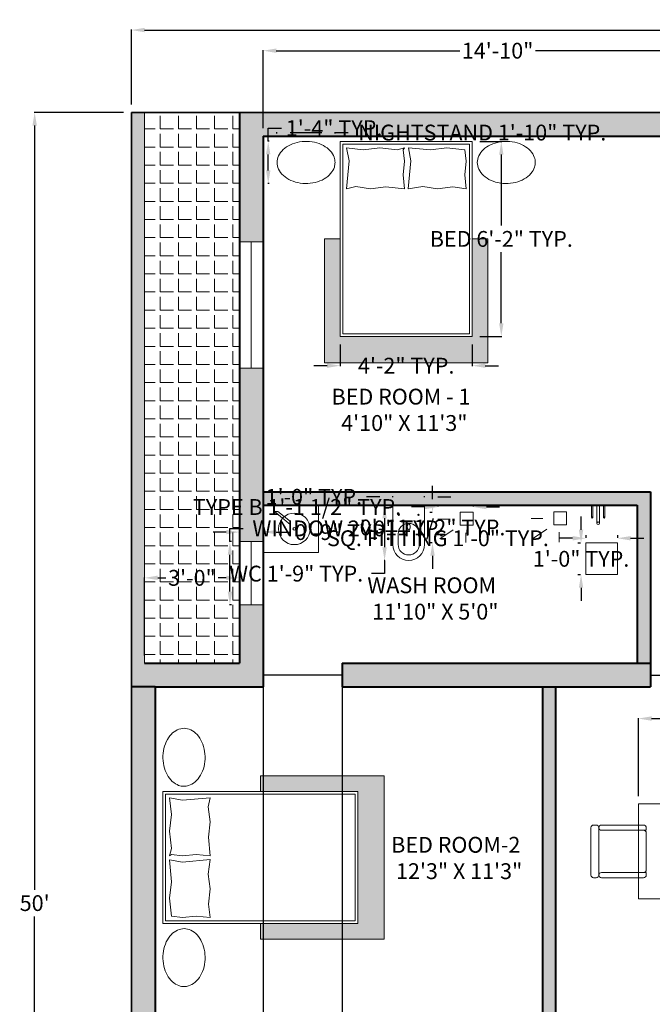
# Model space of a CAD drawing. Units: inches. Extents: x 242 to 808, y 202 to 873.
# Tile 2 of 3: x 242 to 482, y 500 to 873. Entities that reach past the tile are written whole.
import ezdxf

# ---------------------------------------------------------------- set-up
doc = ezdxf.new("R2010")
doc.units = ezdxf.units.IN
doc.header["$MEASUREMENT"] = 0
for name, color, linetype, lineweight in [('A-ANNO-DIMS', 2, 'Continuous', 18), ('A-AREA-IDEN', 7, 'Continuous', 25), ('A-DOOR', 3, 'Continuous', 25), ('A-FLOR-FIXT', 8, 'Continuous', 18), ('A-FURN', 8, 'Continuous', 18), ('A-FURN-PATT', 253, 'Continuous', 13), ('A-GLAZ', 4, 'Continuous', 18), ('A-SITE-PVMT', 8, 'Continuous', 18), ('A-SITE-PVMT-PATT', 254, 'Continuous', 13), ('A-WALL', 7, 'Continuous', 40), ('A-WALL-PATT', 30, 'Continuous', 13), ('C-PROP', 7, 'Continuous', 35)]:
    doc.layers.add(name, color=color, linetype=linetype, lineweight=lineweight)
doc.styles.get("Standard").update_dxf_attribs({"font": 'arial.ttf'})
doc.dimstyles.get("Standard").update_dxf_attribs({"dimtxt": 6, "dimasz": 5, "dimexe": 0.18, "dimexo": 3, "dimgap": 2, "dimtad": 0, "dimtih": 1, "dimtoh": 1, "dimdec": 0, "dimzin": 0, "dimdsep": 46, "dimlunit": 3, "dimtxsty": 'Standard', "dimcen": 0.09, "dimadec": 0, "dimazin": 0, "dimtfac": 1, "dimtdec": 0, "dimtofl": 0, "dimtmove": 0, "dimatfit": 3, "dimfxl": 1, "dimtolj": 1, "dimtzin": 0, "dimarcsym": 0})

# ---------------------------------------------------------------- blocks, each defined once
blk = doc.blocks.new('*D7')
at = {"layer": 'A-ANNO-DIMS', "color": 0, "lineweight": -2, "transparency": 16777216}
for p, q in [((284.66, 841.15), (284.66, 869.56)), ((289.66, 869.38), (517.45, 869.38)), ((759.66, 869.38), (531.88, 869.38)), ((764.66, 841.15), (764.66, 869.56))]:
    blk.add_line(p, q, dxfattribs=at)
at = {"layer": 'A-ANNO-DIMS', "color": 0, "transparency": 16777216}
for points in [[(289.66, 870.21), (289.66, 868.54), (284.66, 869.38)], [(759.66, 870.21), (759.66, 868.54), (764.66, 869.38)]]:
    blk.add_solid(points, dxfattribs=at)
at = {"layer": 'Defpoints', "color": 0, "transparency": 16777216}
for p in [(764.66, 869.38), (284.66, 838.15), (764.66, 838.15)]:
    blk.add_point(p, dxfattribs=at)
at = {"layer": 'A-ANNO-DIMS', "color": 0, "transparency": 16777216, "insert": (524.66, 869.38), "char_height": 6, "attachment_point": 5}
blk.add_mtext("\\A1;40'", dxfattribs=at)
blk = doc.blocks.new('*D8')
at = {"layer": 'A-ANNO-DIMS', "color": 0, "lineweight": -2, "transparency": 16777216}
for p, q in [((281.66, 838.15), (247.79, 838.15)), ((247.97, 833.15), (247.97, 543.22)), ((247.97, 243.15), (247.97, 533.09)), ((281.66, 238.15), (247.79, 238.15))]:
    blk.add_line(p, q, dxfattribs=at)
at = {"layer": 'A-ANNO-DIMS', "color": 0, "transparency": 16777216}
for points in [[(247.13, 833.15), (248.8, 833.15), (247.97, 838.15)], [(247.13, 243.15), (248.8, 243.15), (247.97, 238.15)]]:
    blk.add_solid(points, dxfattribs=at)
at = {"layer": 'Defpoints', "color": 0, "transparency": 16777216}
for p in [(284.66, 838.15), (247.97, 238.15), (284.66, 238.15)]:
    blk.add_point(p, dxfattribs=at)
at = {"layer": 'A-ANNO-DIMS', "color": 0, "transparency": 16777216, "insert": (247.97, 538.15), "char_height": 6, "attachment_point": 5}
blk.add_mtext("\\A1;50'", dxfattribs=at)
blk = doc.blocks.new('DINING-CHAIR')
for p, q in [((2, 18), (2, 20)), ((3, 21), (17, 21)), ((18, 21), (18, 18)), ((19, 21), (18, 21)), ((18, 20), (18, 18)), ((20, 4), (20, 20)), ((1, 0), (10, 0)), ((10, 0), (19, 0))]:
    blk.add_line(p, q)
for points in [[(0, 1), (0, 2, -0.414214), (1, 3), (1, 3, 0.414214), (2, 4), (2, 21), (1, 21, 0.414214), (0, 20), (0, 4, 0.414214), (1, 3), (19, 3)], [(18, 18), (18, 4, 0.414214), (19, 3), (19, 3, -0.414214), (20, 2), (20, 1)]]:
    blk.add_lwpolyline(points, format="xyb")
for centre, start, end in [((3, 20), 90, 180), ((17, 20), 0, 90), ((19, 20), 0, 90), ((19, 4), 270, 0), ((1, 1), 180, 270), ((19, 1), 270, 0)]:
    blk.add_arc(centre, 1, start, end)
blk = doc.blocks.new('BED-DOUBLE')
for p, q in [((2.42, 71.51), (8.74, 70.74)), ((3.32, 66.6), (2.42, 71.51)), ((2.42, 71.51), (2.42, 71.51)), ((8.74, 70.74), (15, 71.51)), ((15, 71.51), (21.65, 70.74)), ((21.65, 70.74), (24.42, 71.51)), ((24.42, 71.51), (23.82, 70.81)), ((25.88, 71.51), (34.2, 70.74)), ((26.78, 66.6), (25.88, 71.51)), ((25.88, 71.51), (25.88, 71.51)), ((34.2, 70.74), (40.46, 71.51)), ((40.46, 71.51), (47.28, 70.81)), ((23.82, 70.81), (24.35, 66.53)), ((47.28, 70.81), (47.81, 66.53)), ((2.35, 56.03), (3.32, 66.6)), ((24.35, 66.53), (23.85, 61.36)), ((25.81, 56.03), (26.78, 66.6)), ((47.81, 66.53), (47.32, 61.36)), ((23.85, 61.36), (24.35, 56.03)), ((47.32, 61.36), (47.81, 56.03)), ((5.85, 56.87), (2.35, 56.03)), ((11.48, 56.03), (5.85, 56.87)), ((17.24, 56.78), (11.48, 56.03)), ((24.35, 56.03), (17.24, 56.78)), ((31.31, 56.87), (25.81, 56.03)), ((36.94, 56.03), (31.31, 56.87)), ((42.7, 56.78), (36.94, 56.03)), ((47.81, 56.03), (42.7, 56.78))]:
    blk.add_line(p, q)
for points in [[(0, 74), (50, 74), (50, 0), (0, 0)], [(1, 73), (49, 73), (49, 1), (1, 1)]]:
    blk.add_lwpolyline(points, close=True)
blk = doc.blocks.new('BEDSIDE-TABLE')
blk.add_open_spline([(22, 8), (22, 8.68), (21.88, 9.37), (21.33, 10.88), (20.82, 11.7), (19.44, 13.19), (18.57, 13.86), (16.55, 14.96), (15.4, 15.38), (12.98, 15.92), (11.7, 16.04), (9.16, 15.94), (7.91, 15.73), (5.57, 15.01), (4.5, 14.5), (2.65, 13.27), (1.88, 12.54), (0.72, 10.97), (0.33, 10.13), (-0.05, 8.41), (-0.05, 7.54), (0.35, 5.81), (0.76, 4.96), (1.95, 3.37), (2.75, 2.64), (4.64, 1.41), (5.75, 0.92), (8.13, 0.22), (9.41, 0.03), (11.98, -0.02), (13.27, 0.12), (15.7, 0.71), (16.84, 1.17), (18.83, 2.32), (19.68, 3.02), (21, 4.56), (21.47, 5.4), (21.91, 6.84), (22, 7.42), (22, 8)], degree=3, knots=[0, 0, 0, 0, 0.267442, 0.267442, 0.605946, 0.605946, 0.944449, 0.944449, 1.282952, 1.282952, 1.621455, 1.621455, 1.959959, 1.959959, 2.298462, 2.298462, 2.636965, 2.636965, 2.975469, 2.975469, 3.313972, 3.313972, 3.656728, 3.656728, 3.999485, 3.999485, 4.342242, 4.342242, 4.684998, 4.684998, 5.027755, 5.027755, 5.370511, 5.370511, 5.713268, 5.713268, 6.056024, 6.056024, 6.283185, 6.283185, 6.283185, 6.283185])
blk = doc.blocks.new('LAVATORY-VANITY')
for p, q in [((15.59, 16.67), (10.6, 10.67)), ((11.73, 10.63), (15.59, 15.35)), ((15.59, 16.67), (15.59, 15.35)), ((10.6, 10.67), (11.73, 10.63))]:
    blk.add_line(p, q)
blk.add_lwpolyline([(0, 21), (18, 21), (18, 0), (0, 0)], close=True)
for radius in [6, 0.5]:
    blk.add_circle((8.99, 9.16), radius)
blk = doc.blocks.new('WC-PAN')
for p, q in [((0, 15), (0, 0)), ((12, 0), (12, 15)), ((2, 14.93), (2, 10.93)), ((10, 14.93), (10, 10.93))]:
    blk.add_line(p, q)
for centre, radius, start, end in [((6, 15), 6, 0, 180), ((6, 14.93), 4, 0, 180), ((6, 10.93), 4, 180, 0)]:
    blk.add_arc(centre, radius, start, end)
blk.add_ellipse((6, 8.26), major_axis=(0, 1.09), ratio=0.500408)
blk = doc.blocks.new('SHOWER-MIXER')
for p, q in [((0, 4.4), (0, 0)), ((0.5, 4.4), (0.5, 0)), ((2, 6.9), (2, 0)), ((3, 6.9), (3, 0)), ((4.5, 4.4), (4.5, 0)), ((5, 4.4), (5, 0))]:
    blk.add_line(p, q)
for centre, radius in [((0.25, 4.65), 0.25), ((2.5, 6.9), 0.5), ((4.75, 4.65), 0.25)]:
    blk.add_circle(centre, radius)
blk = doc.blocks.new('BATH-FITTING-B')
for p, q in [((2.85, 7.76), (2.85, 11.5)), ((7.55, 6.61), (12.62, 10.02)), ((9.01, 2.54), (13.42, 2.54))]:
    blk.add_line(p, q)
blk.add_lwpolyline([(0, 4.89), (4.89, 4.89), (4.89, 0), (0, 0)], close=True)
blk = doc.blocks.new('WIN-24IN')
blk.add_line((4.5, 24), (4.5, 0))
blk.add_lwpolyline([(0, 24), (9, 24), (9, 0), (0, 0)], close=True)
blk = doc.blocks.new('WIN-48IN')
blk.add_line((4.5, 48), (4.5, 0))
blk.add_lwpolyline([(0, 48), (9, 48), (9, 0), (0, 0)], close=True)
blk = doc.blocks.new('DOOR-30IN-PLAN')
blk.add_line((0, 30), (0, 0))
blk = doc.blocks.new('BATH-FITTING-12IN-SQ')
blk.add_lwpolyline([(0, 12), (12, 12), (12, 0), (0, 0)], close=True)
blk = doc.blocks.new('*D21')
at = {"layer": 'A-ANNO-DIMS', "color": 0, "lineweight": -2, "transparency": 16777216}
for p, q in [((416.96, 827.14), (425.24, 827.14)), ((425.06, 822.14), (425.06, 795.21)), ((425.06, 758.14), (425.06, 785.08)), ((416.96, 753.14), (425.24, 753.14))]:
    blk.add_line(p, q, dxfattribs=at)
at = {"layer": 'A-ANNO-DIMS', "color": 0, "transparency": 16777216}
for points in [[(424.22, 822.14), (425.89, 822.14), (425.06, 827.14)], [(424.22, 758.14), (425.89, 758.14), (425.06, 753.14)]]:
    blk.add_solid(points, dxfattribs=at)
at = {"layer": 'Defpoints', "color": 0, "transparency": 16777216}
for p in [(413.96, 827.14), (425.06, 827.14), (413.96, 753.14)]:
    blk.add_point(p, dxfattribs=at)
at = {"layer": 'A-ANNO-DIMS', "color": 0, "transparency": 16777216, "insert": (425.06, 790.14), "char_height": 6, "attachment_point": 5}
blk.add_mtext('\\A1;BED 6\'-2" TYP.', dxfattribs=at)
blk = doc.blocks.new('*D22')
at = {"layer": 'A-ANNO-DIMS', "color": 0, "lineweight": -2, "transparency": 16777216}
for p, q in [((363.96, 750.14), (363.96, 741.86)), ((413.96, 750.14), (413.96, 741.86)), ((358.96, 742.04), (353.96, 742.04)), ((418.96, 742.04), (423.96, 742.04))]:
    blk.add_line(p, q, dxfattribs=at)
at = {"layer": 'A-ANNO-DIMS', "color": 0, "transparency": 16777216}
for points in [[(358.96, 742.88), (358.96, 741.21), (363.96, 742.04)], [(418.96, 742.88), (418.96, 741.21), (413.96, 742.04)]]:
    blk.add_solid(points, dxfattribs=at)
at = {"layer": 'Defpoints', "color": 0, "transparency": 16777216}
for p in [(363.96, 753.14), (413.96, 753.14), (413.96, 742.04)]:
    blk.add_point(p, dxfattribs=at)
at = {"layer": 'A-ANNO-DIMS', "color": 0, "transparency": 16777216, "insert": (388.96, 742.04), "char_height": 6, "attachment_point": 5}
blk.add_mtext('\\A1;4\'-2" TYP.', dxfattribs=at)
blk = doc.blocks.new('*D23')
at = {"layer": 'A-ANNO-DIMS', "color": 0, "lineweight": -2, "transparency": 16777216}
for p, q in [((339.9, 830.18), (339.9, 830.67)), ((344.9, 830.49), (356.96, 830.49)), ((361.96, 830.18), (361.96, 830.67)), ((361.96, 830.49), (366.96, 830.49))]:
    blk.add_line(p, q, dxfattribs=at)
at = {"layer": 'A-ANNO-DIMS', "color": 0, "transparency": 16777216}
for points in [[(344.9, 831.33), (344.9, 829.66), (339.9, 830.49)], [(356.96, 831.33), (356.96, 829.66), (361.96, 830.49)]]:
    blk.add_solid(points, dxfattribs=at)
at = {"layer": 'Defpoints', "color": 0, "transparency": 16777216}
for p in [(361.96, 830.49), (339.9, 827.18), (361.96, 827.18)]:
    blk.add_point(p, dxfattribs=at)
at = {"layer": 'A-ANNO-DIMS', "color": 0, "transparency": 16777216, "insert": (417.83, 830.49), "char_height": 6, "attachment_point": 5}
blk.add_mtext('\\A1;NIGHTSTAND 1\'-10" TYP.', dxfattribs=at)
blk = doc.blocks.new('*D24')
at = {"layer": 'A-ANNO-DIMS', "color": 0, "lineweight": -2, "transparency": 16777216}
for p, q in [((336.6, 827.18), (336.6, 832.18)), ((336.6, 832.18), (341.6, 832.18)), ((336.9, 827.18), (336.42, 827.18)), ((336.6, 816.12), (336.6, 822.18)), ((336.9, 811.12), (336.42, 811.12))]:
    blk.add_line(p, q, dxfattribs=at)
at = {"layer": 'A-ANNO-DIMS', "color": 0, "transparency": 16777216}
for points in [[(335.76, 822.18), (337.43, 822.18), (336.6, 827.18)], [(335.76, 816.12), (337.43, 816.12), (336.6, 811.12)]]:
    blk.add_solid(points, dxfattribs=at)
at = {"layer": 'Defpoints', "color": 0, "transparency": 16777216}
for p in [(336.6, 827.18), (339.9, 827.18), (339.9, 811.12)]:
    blk.add_point(p, dxfattribs=at)
at = {"layer": 'A-ANNO-DIMS', "color": 0, "transparency": 16777216, "insert": (361.6, 832.18), "char_height": 6, "attachment_point": 5}
blk.add_mtext('\\A1;1\'-4" TYP.', dxfattribs=at)
blk = doc.blocks.new('*D29')
at = {"layer": 'A-ANNO-DIMS', "color": 0, "lineweight": -2, "transparency": 16777216}
for p, q in [((380.91, 689.15), (380.58, 689.15)), ((380.76, 684.15), (380.76, 673.15)), ((380.91, 668.15), (380.58, 668.15)), ((380.76, 668.15), (380.76, 663.15)), ((380.76, 663.15), (375.76, 663.15))]:
    blk.add_line(p, q, dxfattribs=at)
at = {"layer": 'A-ANNO-DIMS', "color": 0, "transparency": 16777216}
for points in [[(379.93, 684.15), (381.6, 684.15), (380.76, 689.15)], [(379.93, 673.15), (381.6, 673.15), (380.76, 668.15)]]:
    blk.add_solid(points, dxfattribs=at)
at = {"layer": 'Defpoints', "color": 0, "transparency": 16777216}
for p in [(383.91, 689.15), (380.76, 668.15), (383.91, 668.15)]:
    blk.add_point(p, dxfattribs=at)
at = {"layer": 'A-ANNO-DIMS', "color": 0, "transparency": 16777216, "insert": (347.21, 663.15), "char_height": 6, "attachment_point": 5}
blk.add_mtext('\\A1;WC 1\'-9" TYP.', dxfattribs=at)
blk = doc.blocks.new('*D30')
at = {"layer": 'A-ANNO-DIMS', "color": 0, "lineweight": -2, "transparency": 16777216}
for p, q in [((378.91, 692.3), (373.91, 692.3)), ((383.91, 692.15), (383.91, 692.48)), ((395.91, 692.15), (395.91, 692.48)), ((400.91, 692.3), (405.91, 692.3))]:
    blk.add_line(p, q, dxfattribs=at)
at = {"layer": 'A-ANNO-DIMS', "color": 0, "transparency": 16777216}
for points in [[(378.91, 693.14), (378.91, 691.47), (383.91, 692.3)], [(400.91, 693.14), (400.91, 691.47), (395.91, 692.3)]]:
    blk.add_solid(points, dxfattribs=at)
at = {"layer": 'Defpoints', "color": 0, "transparency": 16777216}
for p in [(383.91, 692.3), (383.91, 689.15), (395.91, 689.15)]:
    blk.add_point(p, dxfattribs=at)
at = {"layer": 'A-ANNO-DIMS', "color": 0, "transparency": 16777216, "insert": (353.91, 692.3), "char_height": 6, "attachment_point": 5}
blk.add_mtext('\\A1;1\'-0" TYP.', dxfattribs=at)
blk = doc.blocks.new('*D35')
at = {"layer": 'A-ANNO-DIMS', "color": 0, "lineweight": -2, "transparency": 16777216}
for p, q in [((395.97, 688.43), (390.97, 688.43)), ((400.97, 689.42), (400.97, 688.61)), ((414.39, 689.42), (414.39, 688.61)), ((419.39, 688.43), (424.39, 688.43))]:
    blk.add_line(p, q, dxfattribs=at)
at = {"layer": 'A-ANNO-DIMS', "color": 0, "transparency": 16777216}
for points in [[(395.97, 689.26), (395.97, 687.59), (400.97, 688.43)], [(419.39, 689.26), (419.39, 687.59), (414.39, 688.43)]]:
    blk.add_solid(points, dxfattribs=at)
at = {"layer": 'Defpoints', "color": 0, "transparency": 16777216}
for p in [(400.97, 688.43), (400.97, 686.42), (414.39, 686.42)]:
    blk.add_point(p, dxfattribs=at)
at = {"layer": 'A-ANNO-DIMS', "color": 0, "transparency": 16777216, "insert": (347.54, 688.43), "char_height": 6, "attachment_point": 5}
blk.add_mtext('\\A1;TYPE B 1\'-1 1/2" TYP.', dxfattribs=at)
blk = doc.blocks.new('*D36')
at = {"layer": 'A-ANNO-DIMS', "color": 0, "lineweight": -2, "transparency": 16777216}
for p, q in [((398.95, 691.42), (398.95, 696.42)), ((397.97, 686.42), (398.77, 686.42)), ((397.97, 674.91), (398.77, 674.91)), ((398.95, 669.91), (398.95, 664.91))]:
    blk.add_line(p, q, dxfattribs=at)
at = {"layer": 'A-ANNO-DIMS', "color": 0, "transparency": 16777216}
for points in [[(398.12, 691.42), (399.79, 691.42), (398.95, 686.42)], [(398.12, 669.91), (399.79, 669.91), (398.95, 674.91)]]:
    blk.add_solid(points, dxfattribs=at)
at = {"layer": 'Defpoints', "color": 0, "transparency": 16777216}
for p in [(400.97, 686.42), (398.95, 674.91), (400.97, 674.91)]:
    blk.add_point(p, dxfattribs=at)
at = {"layer": 'A-ANNO-DIMS', "color": 0, "transparency": 16777216, "insert": (398.95, 680.66), "char_height": 6, "attachment_point": 5}
blk.add_mtext('\\A1;0\'-11 1/2" TYP.', dxfattribs=at)
blk = doc.blocks.new('*D37')
at = {"layer": 'A-ANNO-DIMS', "color": 0, "lineweight": -2, "transparency": 16777216}
for p, q in [((452.13, 676.57), (447.13, 676.57)), ((457.13, 677.77), (457.13, 676.75)), ((469.13, 677.77), (469.13, 676.75)), ((474.13, 676.57), (479.13, 676.57))]:
    blk.add_line(p, q, dxfattribs=at)
at = {"layer": 'A-ANNO-DIMS', "color": 0, "transparency": 16777216}
for points in [[(452.13, 677.4), (452.13, 675.74), (457.13, 676.57)], [(474.13, 677.4), (474.13, 675.74), (469.13, 676.57)]]:
    blk.add_solid(points, dxfattribs=at)
at = {"layer": 'Defpoints', "color": 0, "transparency": 16777216}
for p in [(457.13, 676.57), (457.13, 674.77), (469.13, 674.77)]:
    blk.add_point(p, dxfattribs=at)
at = {"layer": 'A-ANNO-DIMS', "color": 0, "transparency": 16777216, "insert": (401.01, 676.57), "char_height": 6, "attachment_point": 5}
blk.add_mtext('\\A1;SQ. FITTING 1\'-0" TYP.', dxfattribs=at)
blk = doc.blocks.new('*D38')
at = {"layer": 'A-ANNO-DIMS', "color": 0, "lineweight": -2, "transparency": 16777216}
for p, q in [((455.33, 679.77), (455.33, 684.77)), ((454.13, 674.77), (455.15, 674.77)), ((454.13, 662.77), (455.15, 662.77)), ((455.33, 657.77), (455.33, 652.77))]:
    blk.add_line(p, q, dxfattribs=at)
at = {"layer": 'A-ANNO-DIMS', "color": 0, "transparency": 16777216}
for points in [[(454.49, 679.77), (456.16, 679.77), (455.33, 674.77)], [(454.49, 657.77), (456.16, 657.77), (455.33, 662.77)]]:
    blk.add_solid(points, dxfattribs=at)
at = {"layer": 'Defpoints', "color": 0, "transparency": 16777216}
for p in [(457.13, 674.77), (455.33, 662.77), (457.13, 662.77)]:
    blk.add_point(p, dxfattribs=at)
at = {"layer": 'A-ANNO-DIMS', "color": 0, "transparency": 16777216, "insert": (455.33, 668.77), "char_height": 6, "attachment_point": 5}
blk.add_mtext('\\A1;1\'-0" TYP.', dxfattribs=at)
blk = doc.blocks.new('*D39')
at = {"layer": 'A-ANNO-DIMS', "color": 0, "lineweight": -2, "transparency": 16777216}
for p, q in [((322.06, 675.31), (322.06, 680.31)), ((322.06, 680.31), (327.06, 680.31)), ((322.66, 675.31), (321.88, 675.31)), ((322.06, 656.31), (322.06, 670.31)), ((322.66, 651.31), (321.88, 651.31))]:
    blk.add_line(p, q, dxfattribs=at)
at = {"layer": 'A-ANNO-DIMS', "color": 0, "transparency": 16777216}
for points in [[(321.23, 670.31), (322.9, 670.31), (322.06, 675.31)], [(321.23, 656.31), (322.9, 656.31), (322.06, 651.31)]]:
    blk.add_solid(points, dxfattribs=at)
at = {"layer": 'Defpoints', "color": 0, "transparency": 16777216}
for p in [(322.06, 675.31), (325.66, 675.31), (325.66, 651.31)]:
    blk.add_point(p, dxfattribs=at)
at = {"layer": 'A-ANNO-DIMS', "color": 0, "transparency": 16777216, "insert": (367.03, 680.31), "char_height": 6, "attachment_point": 5}
blk.add_mtext('\\A1;WINDOW 2\'-0" TYP.', dxfattribs=at)
blk = doc.blocks.new('*D40')
at = {"layer": 'A-ANNO-DIMS', "color": 0, "lineweight": -2, "transparency": 16777216}
for p, q in [((320.66, 678.91), (315.66, 678.91)), ((325.66, 678.31), (325.66, 679.09)), ((334.66, 678.31), (334.66, 679.09)), ((339.66, 678.91), (344.66, 678.91))]:
    blk.add_line(p, q, dxfattribs=at)
at = {"layer": 'A-ANNO-DIMS', "color": 0, "transparency": 16777216}
for points in [[(320.66, 679.75), (320.66, 678.08), (325.66, 678.91)], [(339.66, 679.75), (339.66, 678.08), (334.66, 678.91)]]:
    blk.add_solid(points, dxfattribs=at)
at = {"layer": 'Defpoints', "color": 0, "transparency": 16777216}
for p in [(334.66, 678.91), (325.66, 675.31), (334.66, 675.31)]:
    blk.add_point(p, dxfattribs=at)
at = {"layer": 'A-ANNO-DIMS', "color": 0, "transparency": 16777216, "insert": (364.95, 678.91), "char_height": 6, "attachment_point": 5}
blk.add_mtext('\\A1;0\'-9" TYP.', dxfattribs=at)
blk = doc.blocks.new('*D43')
at = {"layer": 'A-ANNO-DIMS', "color": 0, "lineweight": -2, "transparency": 16777216}
for p, q in [((334.66, 832.15), (334.66, 861.73)), ((339.66, 861.55), (409.31, 861.55)), ((507.66, 861.55), (438.02, 861.55)), ((512.66, 832.15), (512.66, 861.73))]:
    blk.add_line(p, q, dxfattribs=at)
at = {"layer": 'A-ANNO-DIMS', "color": 0, "transparency": 16777216}
for points in [[(339.66, 862.39), (339.66, 860.72), (334.66, 861.55)], [(507.66, 862.39), (507.66, 860.72), (512.66, 861.55)]]:
    blk.add_solid(points, dxfattribs=at)
at = {"layer": 'Defpoints', "color": 0, "transparency": 16777216}
for p in [(512.66, 861.55), (334.66, 829.15), (512.66, 829.15)]:
    blk.add_point(p, dxfattribs=at)
at = {"layer": 'A-ANNO-DIMS', "color": 0, "transparency": 16777216, "insert": (423.66, 861.55), "char_height": 6, "attachment_point": 5}
blk.add_mtext('\\A1;14\'-10"', dxfattribs=at)
blk = doc.blocks.new('*D46')
at = {"layer": 'A-ANNO-DIMS', "color": 0, "lineweight": -2, "transparency": 16777216}
for p, q in [((364.66, 626.15), (364.66, 205.57)), ((334.66, 621.65), (334.66, 205.57)), ((329.66, 205.75), (324.66, 205.75)), ((369.66, 205.75), (374.66, 205.75))]:
    blk.add_line(p, q, dxfattribs=at)
at = {"layer": 'A-ANNO-DIMS', "color": 0, "transparency": 16777216}
for points in [[(329.66, 206.59), (329.66, 204.92), (334.66, 205.75)], [(369.66, 206.59), (369.66, 204.92), (364.66, 205.75)]]:
    blk.add_solid(points, dxfattribs=at)
at = {"layer": 'Defpoints', "color": 0, "transparency": 16777216}
for p in [(364.66, 629.15), (334.66, 624.65), (364.66, 205.75)]:
    blk.add_point(p, dxfattribs=at)
at = {"layer": 'A-ANNO-DIMS', "color": 0, "transparency": 16777216, "insert": (349.66, 205.75), "char_height": 6, "attachment_point": 5}
blk.add_mtext('\\A1;2\'-6"', dxfattribs=at)
blk = doc.blocks.new('*D49')
at = {"layer": 'A-ANNO-DIMS', "color": 0, "lineweight": -2, "transparency": 16777216}
for p, q in [((289.66, 632.15), (289.66, 661.73)), ((294.66, 661.55), (297.69, 661.55)), ((320.66, 661.55), (317.64, 661.55)), ((325.66, 632.15), (325.66, 661.73))]:
    blk.add_line(p, q, dxfattribs=at)
at = {"layer": 'A-ANNO-DIMS', "color": 0, "transparency": 16777216}
for points in [[(294.66, 662.39), (294.66, 660.72), (289.66, 661.55)], [(320.66, 662.39), (320.66, 660.72), (325.66, 661.55)]]:
    blk.add_solid(points, dxfattribs=at)
at = {"layer": 'Defpoints', "color": 0, "transparency": 16777216}
for p in [(325.66, 661.55), (289.66, 629.15), (325.66, 629.15)]:
    blk.add_point(p, dxfattribs=at)
at = {"layer": 'A-ANNO-DIMS', "color": 0, "transparency": 16777216, "insert": (307.66, 661.55), "char_height": 6, "attachment_point": 5}
blk.add_mtext('\\A1;3\'-0"', dxfattribs=at)
blk = doc.blocks.new('*D50')
at = {"layer": 'A-ANNO-DIMS', "color": 0, "lineweight": -2, "transparency": 16777216}
for p, q in [((477.06, 578.76), (477.06, 608.34)), ((482.06, 608.16), (515.08, 608.16)), ((568.06, 608.16), (535.04, 608.16)), ((573.06, 578.76), (573.06, 608.34))]:
    blk.add_line(p, q, dxfattribs=at)
at = {"layer": 'A-ANNO-DIMS', "color": 0, "transparency": 16777216}
for points in [[(482.06, 608.99), (482.06, 607.32), (477.06, 608.16)], [(568.06, 608.99), (568.06, 607.32), (573.06, 608.16)]]:
    blk.add_solid(points, dxfattribs=at)
at = {"layer": 'Defpoints', "color": 0, "transparency": 16777216}
for p in [(573.06, 608.16), (477.06, 575.76), (573.06, 575.76)]:
    blk.add_point(p, dxfattribs=at)
at = {"layer": 'A-ANNO-DIMS', "color": 0, "transparency": 16777216, "insert": (525.06, 608.16), "char_height": 6, "attachment_point": 5}
blk.add_mtext('\\A1;8\'-0"', dxfattribs=at)

msp = doc.modelspace()

# ---------------------------------------------------------------- hatches: boundary and pattern name
at = {"layer": 'A-FURN-PATT'}
h = msp.add_hatch(dxfattribs=at)
h.set_pattern_fill('AR-SAND', color=256, scale=2, angle=180)
h.paths.add_polyline_path([(380.66, 586.46), (333.66, 586.46), (333.66, 580.46), (370.66, 580.46), (370.66, 530.46), (333.66, 530.46), (333.66, 524.46), (370.66, 524.46), (380.66, 524.46)])
h.paths.add_polyline_path([(419.96, 753.14), (419.96, 790.14), (413.96, 790.14), (413.96, 753.14), (363.95, 753.14), (363.95, 790.14), (357.96, 790.14), (357.96, 743.14), (419.96, 743.14)])
at = {"layer": 'A-SITE-PVMT-PATT'}
h = msp.add_hatch(dxfattribs=at)
h.set_pattern_fill('ANGLE', color=256, scale=25)
h.set_pattern_definition([(0, (0, 0), (0, 6.875), [5, -1.875]), (90, (0, 0), (-6.875, 4e-16), [5, -1.875])])
h.paths.add_polyline_path([(325.66, 838.15), (289.66, 838.15), (289.66, 629.15), (325.66, 629.15)])
at = {"layer": 'A-WALL-PATT'}
h = msp.add_hatch(color=256, dxfattribs=at)
h.dxf.hatch_style = 1
h.paths.add_polyline_path([(521.66, 838.15), (325.66, 838.15), (325.66, 789.05), (334.66, 789.05), (334.66, 829.15), (512.66, 829.15), (512.66, 788.15), (714.66, 788.15), (723.66, 788.15), (723.66, 797.15), (521.66, 797.15)])
h.paths.add_polyline_path([(764.66, 838.15), (521.66, 838.15), (521.66, 833.15), (759.66, 833.15), (759.66, 629.15), (764.66, 629.15)])
h.paths.add_polyline_path([(723.66, 788.15), (714.66, 788.15), (714.66, 767.17), (723.66, 767.17)], flags=17)
h.paths.add_polyline_path([(723.66, 743.17), (714.66, 743.17), (714.66, 721.15), (622.66, 721.15), (622.66, 758.15), (617.66, 758.15), (617.66, 721.15), (521.66, 721.15), (521.66, 716.15), (643.66, 716.15), (643.66, 659.15), (648.66, 659.15), (648.66, 716.15), (714.66, 716.15), (714.66, 688.28), (723.66, 688.28)], flags=17)
h.paths.add_polyline_path([(764.66, 629.15), (759.66, 629.15), (723.66, 629.15), (723.66, 664.28), (714.66, 664.28), (714.66, 629.15), (648.66, 629.15), (643.66, 629.15), (643.66, 620.15), (759.66, 620.15), (759.66, 403.15), (759.66, 398.15), (759.66, 238.15), (764.66, 238.15)])
h.paths.add_polyline_path([(521.66, 758.15), (512.66, 758.15), (512.66, 620.15), (521.66, 620.15)])
h.paths.add_polyline_path([(481.66, 694.15), (334.66, 694.15), (334.66, 689.15), (476.66, 689.15), (476.66, 629.15), (481.66, 629.15)])
h.paths.add_polyline_path([(334.66, 741.05), (325.66, 741.05), (325.66, 675.31), (334.66, 675.31), (334.66, 689.15), (334.66, 694.15)], flags=17)
h.paths.add_polyline_path([(334.66, 651.31), (325.66, 651.31), (325.66, 629.15), (289.66, 629.15), (289.66, 838.15), (284.66, 838.15), (284.66, 620.15), (293.66, 620.15), (334.66, 620.15)])
h.paths.add_polyline_path([(293.66, 620.15), (284.66, 620.15), (284.66, 485.15), (293.66, 485.15)])
h.paths.add_polyline_path([(307.66, 485.15), (293.66, 485.15), (284.66, 485.15), (284.66, 238.15), (615.66, 238.15), (615.66, 243.15), (289.66, 243.15), (289.66, 480.15), (307.66, 480.15)])
h.paths.add_polyline_path([(373.66, 485.15), (355.66, 485.15), (355.66, 480.15), (373.66, 480.15)], flags=17)
h.paths.add_polyline_path([(445.66, 620.15), (440.66, 620.15), (440.66, 485.15), (373.66, 485.15), (373.66, 480.15), (373.66, 415.15), (410.66, 415.15), (410.66, 420.15), (378.66, 420.15), (378.66, 480.15), (440.66, 480.15), (440.66, 415.15), (445.66, 415.15)])
h.paths.add_polyline_path([(472.95, 336.15), (444.15, 336.15), (444.15, 327.15), (472.95, 327.15)], flags=17)
h.paths.add_polyline_path([(543.66, 485.15), (481.66, 485.15), (481.66, 480.15), (534.66, 480.15), (534.66, 336.15), (520.95, 336.15), (520.95, 327.15), (543.66, 327.15)], flags=17)
h.paths.add_polyline_path([(699.66, 456.15), (649.16, 456.15), (649.16, 451.15), (694.66, 451.15), (694.66, 398.15), (759.66, 398.15), (759.66, 403.15), (699.66, 403.15)], flags=17)
h.paths.add_polyline_path([(481.66, 629.15), (476.66, 629.15), (364.66, 629.15), (364.66, 620.15), (481.66, 620.15)])

# ---------------------------------------------------------------- linework, layer by layer
at = {"layer": 'A-DOOR'}
msp.add_line((481.66, 624.65), (512.66, 624.65), dxfattribs=at)
at = {"layer": 'A-FLOR-FIXT'}
for centre in [(386.22, 685.46), (393.6, 685.46)]:
    msp.add_circle(centre, 0.25, dxfattribs=at)
at = {"layer": 'A-FURN'}
for p, q in [((363.95, 790.14), (357.96, 790.14)), ((357.96, 790.14), (357.96, 743.14)), ((413.96, 790.14), (419.96, 790.14)), ((419.96, 790.14), (419.96, 753.14)), ((419.96, 753.14), (419.96, 743.14)), ((419.96, 743.14), (357.96, 743.14)), ((333.66, 580.46), (333.66, 586.46)), ((333.66, 586.46), (380.66, 586.46)), ((380.66, 524.46), (380.66, 586.46)), ((333.66, 530.46), (333.66, 524.46)), ((333.66, 524.46), (370.66, 524.46)), ((370.66, 524.46), (380.66, 524.46))]:
    msp.add_line(p, q, dxfattribs=at)
msp.add_lwpolyline([(477.06, 575.76), (573.06, 575.76), (573.06, 539.76), (477.06, 539.76)], close=True, dxfattribs=at)
at = {"layer": 'A-SITE-PVMT'}
msp.add_line((289.66, 838.15), (289.66, 629.15), dxfattribs=at)
at = {"layer": 'A-WALL'}
for p, q in [((325.66, 838.15), (325.66, 629.15)), ((334.66, 829.15), (334.66, 694.15)), ((334.66, 829.15), (512.66, 829.15)), ((334.66, 694.15), (481.66, 694.15)), ((334.66, 694.15), (334.66, 689.15)), ((481.66, 694.15), (481.66, 620.15)), ((334.66, 689.15), (476.66, 689.15)), ((334.66, 689.15), (334.66, 620.15)), ((476.66, 689.15), (476.66, 629.15)), ((289.66, 629.15), (325.66, 629.15)), ((364.66, 629.15), (476.66, 629.15)), ((364.66, 629.15), (364.66, 620.15)), ((476.66, 629.15), (481.66, 629.15)), ((293.66, 620.15), (284.66, 620.15)), ((293.66, 620.15), (334.66, 620.15)), ((293.66, 620.15), (293.66, 485.15)), ((364.66, 620.15), (481.66, 620.15)), ((440.66, 620.15), (440.66, 485.15)), ((445.66, 620.15), (445.66, 415.15))]:
    msp.add_line(p, q, dxfattribs=at)
at = {"layer": 'C-PROP'}
for p, q in [((284.66, 838.15), (764.66, 838.15)), ((284.66, 238.15), (284.66, 838.15))]:
    msp.add_line(p, q, dxfattribs=at)

# ---------------------------------------------------------------- block references
at = {"layer": 'A-DOOR', "rotation": 270}
msp.add_blockref('DOOR-30IN-PLAN', (334.66, 624.65), dxfattribs=at)
at = {"layer": 'A-FLOR-FIXT'}
for name, p, rotation in [('LAVATORY-VANITY', (355.66, 671.15), 90.00000000000028), ('WC-PAN', (395.91, 689.15), 180), ('SHOWER-MIXER', (464.32, 689.15), 180), ('BATH-FITTING-B', (414.39, 686.41), 180), ('BATH-FITTING-B', (449.85, 686.58), 180), ('BATH-FITTING-12IN-SQ', (469.13, 674.77), 180)]:
    msp.add_blockref(name, p, dxfattribs=dict(at, rotation=rotation))
at = {"layer": 'A-FURN'}
for name, p in [('BEDSIDE-TABLE', (339.96, 811.15)), ('BED-DOUBLE', (363.95, 753.14)), ('BEDSIDE-TABLE', (415.95, 811.15))]:
    msp.add_blockref(name, p, dxfattribs=at)
at = {"layer": 'A-FURN', "extrusion": (0, 0, -1), "zscale": -1}
for name, p, rotation in [('BEDSIDE-TABLE', (-312.65, 604.46), 270.0000000010102), ('BED-DOUBLE', (-370.66, 580.46), 270.0000000000005), ('BEDSIDE-TABLE', (-312.66, 528.46), 269.9999999999994)]:
    msp.add_blockref(name, p, dxfattribs=dict(at, rotation=rotation))
at = {"layer": 'A-FURN', "rotation": 270.0000000000017}
msp.add_blockref('DINING-CHAIR', (459.06, 567.76), dxfattribs=at)
at = {"layer": 'A-GLAZ'}
for name, p in [('WIN-48IN', (325.66, 741.05)), ('WIN-24IN', (325.66, 651.31))]:
    msp.add_blockref(name, p, dxfattribs=at)

# ---------------------------------------------------------------- texts
at = {"layer": 'A-AREA-IDEN', "char_height": 6, "attachment_point": 1}
for s, insert in [('BED ROOM - 1 \\P  4\'10" X 11\'3"', (360.63, 733.3)), ('WASH ROOM \\P 11\'10" X 5\'0"', (374.23, 661.72)), ('BED ROOM-2\\P 12\'3" X 11\'3"', (383.26, 563.27))]:
    msp.add_mtext_dynamic_manual_height_columns(s, width=78.0144, gutter_width=1, heights=[0], dxfattribs=dict(at, insert=insert))

# ---------------------------------------------------------------- dimensions: what is measured, and where the dimension line sits
at = {"layer": 'A-ANNO-DIMS'}
for base, p1, p2, override, picture, middle in [((764.66, 869.38), (284.66, 838.15), (764.66, 838.15), {"dimclrd": 0, "dimclre": 0, "dimclrt": 0}, '*D7', (524.66, 869.38)), ((512.66, 861.55), (334.66, 829.15), (512.66, 829.15), {"dimdec": 1, "dimlfac": 1, "dimrnd": 0, "dimzin": 1, "dimdsep": 46, "dimlunit": 4, "dimfrac": 2}, '*D43', (423.66, 861.55)), ((325.66, 661.55), (289.66, 629.15), (325.66, 629.15), {"dimdec": 1, "dimlfac": 1, "dimrnd": 0, "dimzin": 1, "dimdsep": 46, "dimlunit": 4, "dimfrac": 2}, '*D49', (307.66, 661.55)), ((364.66, 205.75), (334.66, 624.65), (364.66, 629.15), {"dimdec": 1, "dimlfac": 1, "dimrnd": 0, "dimzin": 1, "dimdsep": 46, "dimlunit": 4, "dimfrac": 2}, '*D46', (349.66, 205.75)), ((573.06, 608.16), (477.06, 575.76), (573.06, 575.76), {"dimdec": 1, "dimlfac": 1, "dimrnd": 0, "dimzin": 1, "dimdsep": 46, "dimlunit": 4, "dimfrac": 2}, '*D50', (525.06, 608.16))]:
    dim = msp.add_linear_dim(base=base, p1=p1, p2=p2, dimstyle='Standard', override=override, dxfattribs=at)
    dim.commit()
    dim.dimension.update_dxf_attribs({"geometry": picture, "text_midpoint": middle})
for base, p1, p2, text, picture, middle in [((361.96, 830.49), (339.9, 827.18), (361.96, 827.18), 'NIGHTSTAND <> TYP.', '*D23', (417.83, 830.49)), ((413.96, 742.04), (363.95, 753.14), (413.96, 753.14), '<> TYP.', '*D22', (388.96, 742.04)), ((334.66, 678.91), (325.66, 675.31), (334.66, 675.31), '<> TYP.', '*D40', (364.95, 678.91))]:
    dim = msp.add_linear_dim(base=base, p1=p1, p2=p2, text=text, dimstyle='Standard', override={"dimdec": 1, "dimlfac": 1, "dimrnd": 0, "dimzin": 1, "dimdsep": 46, "dimlunit": 4, "dimfrac": 2}, dxfattribs=at)
    dim.commit()
    dim.dimension.update_dxf_attribs({"geometry": picture, "text_midpoint": middle})
for base, p1, p2, angle, text, picture, middle in [((336.6, 827.18), (339.9, 811.12), (339.9, 827.18), 90, '<> TYP.', '*D24', (361.6, 832.18)), ((425.06, 827.14), (413.96, 753.14), (413.96, 827.14), 90, 'BED <> TYP.', '*D21', (425.06, 790.14)), ((400.97, 688.43), (414.39, 686.42), (400.97, 686.42), 180, 'TYPE B <> TYP.', '*D35', (347.54, 688.43)), ((383.91, 692.3), (395.91, 689.15), (383.91, 689.15), 180, '<> TYP.', '*D30', (353.91, 692.3)), ((457.13, 676.57), (469.13, 674.77), (457.13, 674.77), 180, 'SQ. FITTING <> TYP.', '*D37', (401.01, 676.57)), ((398.95, 674.91), (400.97, 686.42), (400.97, 674.91), 270, '<> TYP.', '*D36', (398.95, 680.66)), ((322.06, 675.31), (325.66, 651.31), (325.66, 675.31), 90, 'WINDOW <> TYP.', '*D39', (367.03, 680.31)), ((380.76, 668.15), (383.91, 689.15), (383.91, 668.15), 270, 'WC <> TYP.', '*D29', (347.21, 663.15)), ((455.33, 662.77), (457.13, 674.77), (457.13, 662.77), 270, '<> TYP.', '*D38', (455.33, 668.77))]:
    dim = msp.add_linear_dim(base=base, p1=p1, p2=p2, angle=angle, text=text, dimstyle='Standard', override={"dimdec": 1, "dimlfac": 1, "dimrnd": 0, "dimzin": 1, "dimdsep": 46, "dimlunit": 4, "dimfrac": 2}, dxfattribs=at)
    dim.commit()
    dim.dimension.update_dxf_attribs({"geometry": picture, "text_midpoint": middle})
dim = msp.add_linear_dim(base=(247.97, 238.15), p1=(284.66, 838.15), p2=(284.66, 238.15), angle=90, dimstyle='Standard', override={"dimclrd": 0, "dimclre": 0, "dimclrt": 0}, dxfattribs=at)
dim.commit()
dim.dimension.update_dxf_attribs({"geometry": '*D8', "text_midpoint": (247.97, 538.15)})

doc.saveas('drawing.dxf')
